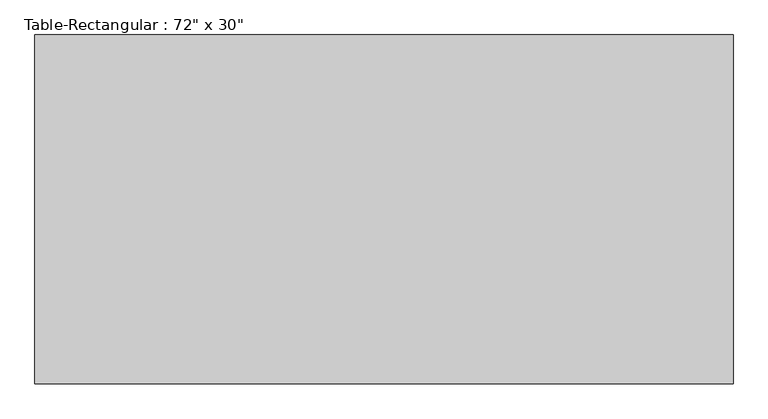
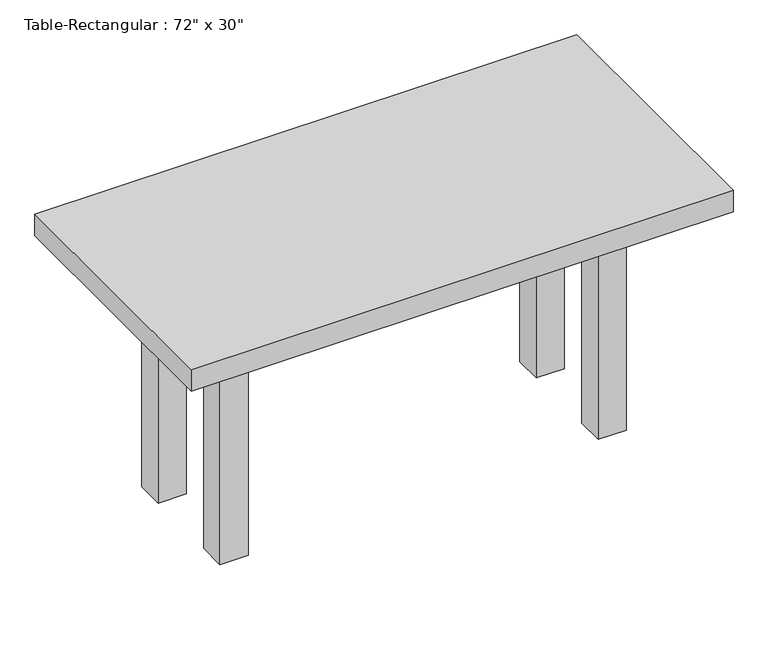
"""IFC4 building model written with IfcOpenShell, lengths in millimetres: furniture geometry."""

from ifc_helpers import new_model, si_unit, frame, origin, origin_with_axes, place, context, project, spatial, polyline, outline, extrude, source, transform, mapped, element, save


def furniture_9a1a9c00(model_context):
    return source(origin(), model_context, "Body", "SweptSolid", [
        extrude(outline(polyline([(393.7, 114.3), (393.7, 88.9), (-393.7, 88.9), (-393.7, 114.3), (393.7, 114.3)])), frame((0.0, 0.0, 457.2), z_axis=(0.0, 0.0, 1.0), x_axis=(1.0, 0.0, 0.0)), (0.0, 0.0, 1.0), 101.6),
        extrude(outline(polyline([(393.7, -114.3), (-393.7, -114.3), (-393.7, -88.9), (393.7, -88.9), (393.7, -114.3)])), frame((0.0, 0.0, 457.2), z_axis=(0.0, 0.0, 1.0), x_axis=(1.0, 0.0, 0.0)), (0.0, 0.0, 1.0), 101.6),
        extrude(outline(polyline([(-406.4, -88.9), (-431.8, -88.9), (-431.8, 88.9), (-406.4, 88.9), (-406.4, -88.9)])), frame((0.0, 0.0, 457.2), z_axis=(0.0, 0.0, 1.0), x_axis=(1.0, 0.0, 0.0)), (0.0, 0.0, 1.0), 101.6),
        extrude(outline(polyline([(406.4, -88.9), (406.4, 88.9), (431.8, 88.9), (431.8, -88.9), (406.4, -88.9)])), frame((0.0, 0.0, 457.2), z_axis=(0.0, 0.0, 1.0), x_axis=(1.0, 0.0, 0.0)), (0.0, 0.0, 1.0), 101.6),
        extrude(outline(polyline([(609.6, 304.8), (609.6, -304.8), (-609.6, -304.8), (-609.6, 304.8), (609.6, 304.8)])), frame((0.0, 0.0, 558.8), z_axis=(0.0, 0.0, 1.0), x_axis=(1.0, 0.0, 0.0)), (0.0, 0.0, 1.0), 50.8),
        extrude(outline(polyline([(-393.7, 152.4), (-393.7, 88.9), (-457.2, 88.9), (-457.2, 152.4), (-393.7, 152.4)])), origin_with_axes(), (0.0, 0.0, 1.0), 558.8),
        extrude(outline(polyline([(393.7, 152.4), (457.2, 152.4), (457.2, 88.9), (393.7, 88.9), (393.7, 152.4)])), origin_with_axes(), (0.0, 0.0, 1.0), 558.8),
        extrude(outline(polyline([(-393.7, -152.4), (-457.2, -152.4), (-457.2, -88.9), (-393.7, -88.9), (-393.7, -152.4)])), origin_with_axes(), (0.0, 0.0, 1.0), 558.8),
        extrude(outline(polyline([(393.7, -152.4), (393.7, -88.9), (457.2, -88.9), (457.2, -152.4), (393.7, -152.4)])), origin_with_axes(), (0.0, 0.0, 1.0), 558.8),
    ])


if __name__ == "__main__":
    model = new_model("IFC4")
    model_context = context("Model", 3, world=origin())
    ifc_project = project(units=[si_unit("LENGTHUNIT", "METRE", prefix="MILLI")], contexts=[model_context])
    site = spatial("IfcSite", under=ifc_project)
    building = spatial("IfcBuilding", under=site)
    placement = place(None, origin())
    furniture_shape = furniture_9a1a9c00(model_context)
    element("IfcFurniture", 1, ObjectType="Table-Rectangular : 72\" x 30\"", at=placement, inside=building, context=model_context, shape_type="MappedRepresentation", body=[
        mapped(furniture_shape, transform((0.0, 0.0, 0.0), x_axis=(1.0, 0.0, 0.0), y_axis=(0.0, 1.0, 0.0), z_axis=(0.0, 0.0, 1.0))),
    ])
    save(model, "model.ifc")

# Revit data of these elements
# Type "Table-Rectangular : 72\" x 30\""
#   Assembly Code = "E2020200"
#   Height = 2' - 0"
#   Length = 4' - 0"
#   Width = 2' - 0"
#   Base Material = Birch
#   Top Material = Birch
#   Default Elevation = 0
# Element 1 (IfcFurniture, "Table-Rectangular : 72\" x 30\"")
#   Materials on its faces: "Birch"
# Materials
#   "Birch": class "Wood", colour RGB 224 178 126, transparency 0, Description = "Betula Alleghaniensis", Cost = 0
